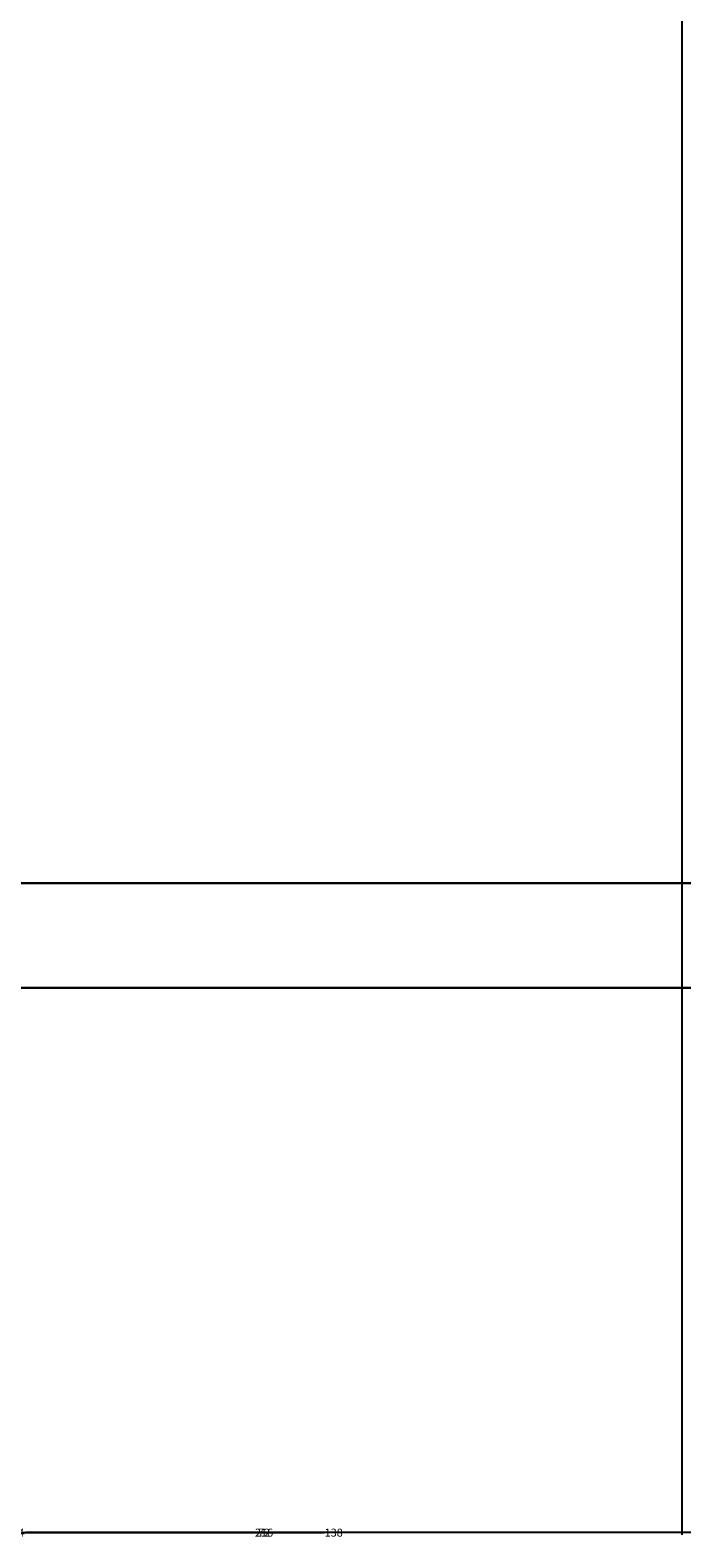
# Model space of a CAD drawing. Units: inches. Extents: x 867 to 1667, y -234 to 788.
# Tile 15 of 42: x 1300 to 1356, y -234 to -104. Entities that reach past the tile are written whole.
import ezdxf

# ---------------------------------------------------------------- set-up
doc = ezdxf.new("R2010")
doc.units = ezdxf.units.IN
doc.header["$MEASUREMENT"] = 0
doc.layers.add('A-ANNO-DIMS', color=2, linetype='Continuous', lineweight=18)
doc.layers.add('A-WALL-SITE', color=8, linetype='Continuous', lineweight=30)
doc.styles.get("Standard").update_dxf_attribs({"font": 'arial.ttf'})
doc.dimstyles.get("Standard").update_dxf_attribs({"dimtxt": 0.6875, "dimasz": 0.18, "dimexe": 0.18, "dimexo": 0.0625, "dimgap": 0.09, "dimtad": 0, "dimdec": 4, "dimzin": 0, "dimdsep": 46, "dimlunit": 4, "dimtxsty": 'Standard', "dimcen": 0.09, "dimadec": 0, "dimazin": 0, "dimtfac": 1, "dimtdec": 4, "dimtofl": 0, "dimtmove": 0, "dimatfit": 3, "dimfxl": 1, "dimtolj": 1, "dimtzin": 0, "dimarcsym": 0})

# ---------------------------------------------------------------- blocks, each defined once
blk = doc.blocks.new('*D27')
at = {"layer": 'A-ANNO-DIMS', "color": 0, "lineweight": -2, "transparency": 16777216}
for p, q in [((1070.89, -55.97), (1070.89, -233.54)), ((1525.26, -186.47), (1525.26, -233.54)), ((1071.07, -233.36), (1296.81, -233.36)), ((1525.08, -233.36), (1299.34, -233.36))]:
    blk.add_line(p, q, dxfattribs=at)
at = {"layer": 'A-ANNO-DIMS', "color": 0, "transparency": 16777216}
for points in [[(1071.07, -233.33), (1071.07, -233.39), (1070.89, -233.36)], [(1525.08, -233.33), (1525.08, -233.39), (1525.26, -233.36)]]:
    blk.add_solid(points, dxfattribs=at)
at = {"layer": 'Defpoints', "color": 0, "transparency": 16777216}
for p in [(1070.89, -55.91), (1525.26, -186.41), (1525.26, -233.36)]:
    blk.add_point(p, dxfattribs=at)
at = {"layer": 'A-ANNO-DIMS', "color": 0, "transparency": 16777216, "insert": (1298.08, -233.36), "char_height": 0.688, "attachment_point": 5}
blk.add_mtext('\\A1;454.4', dxfattribs=at)
blk = doc.blocks.new('*D46')
at = {"layer": 'A-ANNO-DIMS', "color": 0, "lineweight": -2, "transparency": 16777216}
for p, q in [((1256.89, -16.95), (1256.89, -233.54)), ((1394.89, -16.95), (1394.89, -233.54)), ((1257.07, -233.36), (1325.07, -233.36)), ((1394.71, -233.36), (1326.7, -233.36))]:
    blk.add_line(p, q, dxfattribs=at)
at = {"layer": 'A-ANNO-DIMS', "color": 0, "transparency": 16777216}
for points in [[(1257.07, -233.33), (1257.07, -233.39), (1256.89, -233.36)], [(1394.71, -233.33), (1394.71, -233.39), (1394.89, -233.36)]]:
    blk.add_solid(points, dxfattribs=at)
at = {"layer": 'Defpoints', "color": 0, "transparency": 16777216}
for p in [(1256.89, -16.88), (1394.89, -16.88), (1394.89, -233.36)]:
    blk.add_point(p, dxfattribs=at)
at = {"layer": 'A-ANNO-DIMS', "color": 0, "transparency": 16777216, "insert": (1325.89, -233.36), "char_height": 0.688, "attachment_point": 5}
blk.add_mtext('\\A1;138', dxfattribs=at)
blk = doc.blocks.new('*D48')
at = {"layer": 'A-ANNO-DIMS', "color": 0, "lineweight": -2, "transparency": 16777216}
for p, q in [((1283.89, -55.97), (1283.89, -233.54)), ((1355.89, -55.97), (1355.89, -233.54)), ((1284.07, -233.36), (1319.31, -233.36)), ((1355.71, -233.36), (1320.46, -233.36))]:
    blk.add_line(p, q, dxfattribs=at)
at = {"layer": 'A-ANNO-DIMS', "color": 0, "transparency": 16777216}
for points in [[(1284.07, -233.33), (1284.07, -233.39), (1283.89, -233.36)], [(1355.71, -233.33), (1355.71, -233.39), (1355.89, -233.36)]]:
    blk.add_solid(points, dxfattribs=at)
at = {"layer": 'Defpoints', "color": 0, "transparency": 16777216}
for p in [(1283.89, -55.91), (1355.89, -55.91), (1355.89, -233.36)]:
    blk.add_point(p, dxfattribs=at)
at = {"layer": 'A-ANNO-DIMS', "color": 0, "transparency": 16777216, "insert": (1319.89, -233.36), "char_height": 0.688, "attachment_point": 5}
blk.add_mtext('\\A1;72', dxfattribs=at)
blk = doc.blocks.new('*D50')
at = {"layer": 'A-ANNO-DIMS', "color": 0, "lineweight": -2, "transparency": 16777216}
for p, q in [((1211.89, -103.97), (1211.89, -233.54)), ((1427.89, -103.97), (1427.89, -233.54)), ((1212.07, -233.36), (1319.03, -233.36)), ((1427.71, -233.36), (1320.74, -233.36))]:
    blk.add_line(p, q, dxfattribs=at)
at = {"layer": 'A-ANNO-DIMS', "color": 0, "transparency": 16777216}
for points in [[(1212.07, -233.33), (1212.07, -233.39), (1211.89, -233.36)], [(1427.71, -233.33), (1427.71, -233.39), (1427.89, -233.36)]]:
    blk.add_solid(points, dxfattribs=at)
at = {"layer": 'Defpoints', "color": 0, "transparency": 16777216}
for p in [(1211.89, -103.91), (1427.89, -103.91), (1427.89, -233.36)]:
    blk.add_point(p, dxfattribs=at)
at = {"layer": 'A-ANNO-DIMS', "color": 0, "transparency": 16777216, "insert": (1319.89, -233.36), "char_height": 0.688, "attachment_point": 5}
blk.add_mtext('\\A1;216', dxfattribs=at)

msp = doc.modelspace()

# ---------------------------------------------------------------- linework, layer by layer
at = {"layer": 'A-WALL-SITE'}
for p, q in [((1526.8389, -177.4081), (1006.3882, -177.4081)), ((1211.8866, -177.4081), (1427.8866, -177.4081)), ((1619.8866, -186.4081), (914.8866, -186.4081)), ((1211.8866, -186.4081), (1427.8866, -186.4081))]:
    msp.add_line(p, q, dxfattribs=at)

# ---------------------------------------------------------------- dimensions: what is measured, and where the dimension line sits
at = {"layer": 'A-ANNO-DIMS'}
for base, p1, p2, override, picture, middle in [((1394.8866, -233.3581), (1256.8866, -16.883), (1394.8866, -16.883), {"dimdec": 0, "dimlfac": 1, "dimrnd": 0, "dimzin": 0, "dimdsep": 46, "dimlunit": 2}, '*D46', (1325.8866, -233.3581)), ((1525.2648, -233.3581), (1070.8866, -55.9081), (1525.2648, -186.4081), {"dimdec": 1, "dimlfac": 1, "dimrnd": 0, "dimzin": 0, "dimdsep": 46, "dimlunit": 2}, '*D27', (1298.0757, -233.3581)), ((1355.8866, -233.3581), (1283.8866, -55.9081), (1355.8866, -55.9081), {"dimdec": 0, "dimlfac": 1, "dimrnd": 0, "dimzin": 0, "dimdsep": 46, "dimlunit": 2}, '*D48', (1319.8866, -233.3581)), ((1427.8866, -233.3581), (1211.8866, -103.9081), (1427.8866, -103.9081), {"dimdec": 0, "dimlfac": 1, "dimrnd": 0, "dimzin": 0, "dimdsep": 46, "dimlunit": 2}, '*D50', (1319.8866, -233.3581))]:
    dim = msp.add_linear_dim(base=base, p1=p1, p2=p2, dimstyle='Standard', override=override, dxfattribs=at)
    dim.commit()
    dim.dimension.update_dxf_attribs({"geometry": picture, "text_midpoint": middle})

doc.saveas('drawing.dxf')
